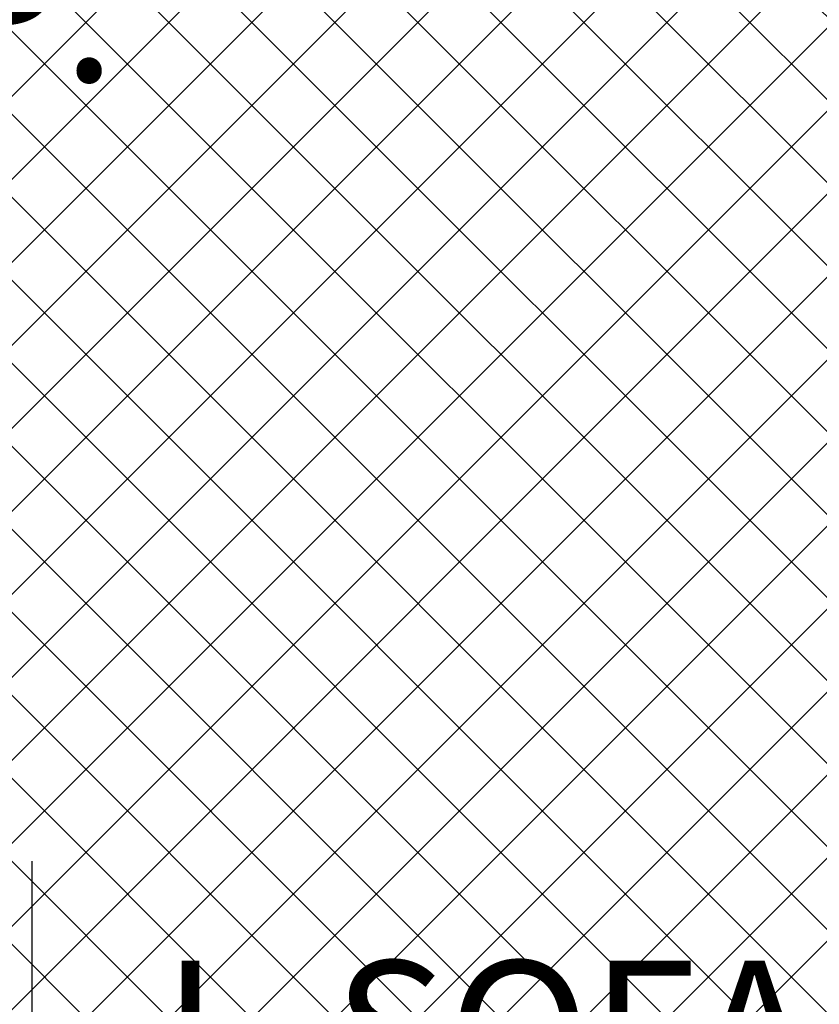
# Model space of a CAD drawing. Units: inches. Extents: x -466983 to 1020, y 324 to 318697.
# Tile 87 of 97: x 742 to 776, y 879 to 921. Entities that reach past the tile are written whole.
import ezdxf

# ---------------------------------------------------------------- set-up
doc = ezdxf.new("R2010")
doc.units = ezdxf.units.IN
doc.header["$MEASUREMENT"] = 0
doc.layers.add('A-ANNO-DIMS', color=2, linetype='Continuous', lineweight=18)
doc.layers.add('A-FLOR-PATT', color=252, linetype='Continuous', lineweight=13)
doc.styles.get("Standard").update_dxf_attribs({"font": 'arial.ttf'})
doc.dimstyles.get("Standard").update_dxf_attribs({"dimtxt": 6, "dimasz": 4, "dimexe": 3, "dimexo": 3, "dimgap": 0.09, "dimtad": 0, "dimtih": 1, "dimtoh": 1, "dimdec": 1, "dimzin": 0, "dimdsep": 46, "dimlunit": 3, "dimtxsty": 'Standard', "dimcen": 0.09, "dimadec": 0, "dimazin": 0, "dimtfac": 1, "dimtdec": 1, "dimtofl": 0, "dimtmove": 0, "dimatfit": 3, "dimfxl": 1, "dimtolj": 1, "dimtzin": 0, "dimarcsym": 0})

# ---------------------------------------------------------------- blocks, each defined once
blk = doc.blocks.new('*D71')
at = {"layer": 'A-ANNO-DIMS', "color": 0, "lineweight": -2, "transparency": 16777216}
for p, q in [((742.215, 885.152), (742.215, 874.91)), ((810.492, 885.152), (810.492, 874.91)), ((738.215, 877.91), (734.215, 877.91)), ((814.492, 877.91), (818.492, 877.91))]:
    blk.add_line(p, q, dxfattribs=at)
at = {"layer": 'A-ANNO-DIMS', "color": 0, "transparency": 16777216}
for points in [[(738.215, 878.577), (738.215, 877.244), (742.215, 877.91)], [(814.492, 878.577), (814.492, 877.244), (810.492, 877.91)]]:
    blk.add_solid(points, dxfattribs=at)
at = {"layer": 'Defpoints', "color": 0, "transparency": 16777216}
for p in [(742.215, 888.152), (810.492, 888.152), (742.215, 877.91)]:
    blk.add_point(p, dxfattribs=at)
at = {"layer": 'A-ANNO-DIMS', "color": 0, "transparency": 16777216, "insert": (776.354, 877.91), "char_height": 6, "attachment_point": 5}
blk.add_mtext('\\A1;L-SOFA 68 TYP.', dxfattribs=at)
blk = doc.blocks.new('*D72')
at = {"layer": 'A-ANNO-DIMS', "color": 0, "lineweight": -2, "transparency": 16777216}
for p, q in [((739.215, 954.575), (728.974, 954.575)), ((731.974, 950.575), (731.974, 924.517)), ((731.974, 892.152), (731.974, 918.21)), ((739.215, 888.152), (728.974, 888.152))]:
    blk.add_line(p, q, dxfattribs=at)
at = {"layer": 'A-ANNO-DIMS', "color": 0, "transparency": 16777216}
for points in [[(731.307, 950.575), (732.641, 950.575), (731.974, 954.575)], [(731.307, 892.152), (732.641, 892.152), (731.974, 888.152)]]:
    blk.add_solid(points, dxfattribs=at)
at = {"layer": 'Defpoints', "color": 0, "transparency": 16777216}
for p in [(731.974, 954.575), (742.215, 954.575), (742.215, 888.152)]:
    blk.add_point(p, dxfattribs=at)
at = {"layer": 'A-ANNO-DIMS', "color": 0, "transparency": 16777216, "insert": (731.974, 921.363), "char_height": 6, "attachment_point": 5}
blk.add_mtext('\\A1;66 TYP.', dxfattribs=at)

msp = doc.modelspace()

# ---------------------------------------------------------------- hatches: boundary and pattern name
at = {"layer": 'A-FLOR-PATT', "transparency": 33554572}
h = msp.add_hatch(dxfattribs=at)
h.set_pattern_fill('ANSI37', color=256, scale=30)
h.set_pattern_definition([(45, (-1212.4137, -290.035), (-2.6516504, 2.6516504), []), (135, (-1212.4137, -290.035), (-2.6516504, -2.6516504), [])])
h.paths.add_polyline_path([(901.806, 1075.938), (900.614, 1075.938), (900.614, 1065.386), (899.391, 1065.386), (898.091, 1065.386), (892.836, 1058.71, -0.258377), (892.188, 1058.351), (879.985, 1058.351, -0.20177), (879.438, 1058.581), (874.081, 1065.386), (872.781, 1065.386), (871.558, 1065.386), (871.558, 1075.938), (813.806, 1075.938), (813.806, 1044.792), (832.395, 1044.792, -0.394795), (848.66, 1028.536), (848.66, 1009.938), (901.806, 1009.938), (901.806, 1015.938), (901.306, 1015.938), (871.306, 1015.938), (871.306, 1017.25), (871.334, 1017.25, -0.401453), (901.306, 1045.938), (901.806, 1045.938)])
edge = h.paths.add_edge_path(flags=16)
edge.add_line((847.773, 1068.949), (847.773, 1073.709))
edge.add_arc((849.227, 1073.709), 1.454, 90, 180, ccw=False)
edge.add_line((849.227, 1075.163), (864.492, 1075.163))
edge.add_arc((864.492, 1073.709), 1.454, 0, 90, ccw=False)
edge.add_line((865.946, 1073.709), (865.946, 1069.004))
edge.add_arc((832.645, 1068.976), 33.301, -20.6123, 0.0472, ccw=False)
edge.add_ellipse((856.859, 1058.48), major_axis=(0, 10.213), ratio=0.685919, start_angle=100.0088, end_angle=259.9912, ccw=False)
edge.add_arc((881.074, 1068.976), 33.301, 180.0472, 200.6123, ccw=False)
h.paths.add_polyline_path([(853.146, 1066.482), (853.146, 1066.453), (853.146, 1066.453, 0.433107), (852.917, 1066.685), (852.917, 1066.453), (853.146, 1066.453), (853.146, 1066.482), (853.088, 1066.612, 0.697939), (852.7, 1066.453), (852.7, 1066.453), (852.7, 1066.482), (852.917, 1067.001), (852.917, 1066.685, -0.396254)], flags=0)
h.paths.add_polyline_path([(861.019, 1066.482), (861.019, 1066.453), (861.019, 1066.453, 0.416404), (860.802, 1066.685), (860.802, 1066.453), (861.019, 1066.453), (861.019, 1066.482), (860.967, 1066.605, 0.713344), (860.573, 1066.453), (860.573, 1066.453), (860.573, 1066.482), (860.802, 1067.001), (860.802, 1066.685, -0.379973)], flags=0)
edge = h.paths.add_edge_path(flags=0)
edge.add_spline(control_points=[(861.13, 1065.785), (861.466, 1065.248), (861.613, 1065.016), (861.983, 1064.374), (862.192, 1063.944), (862.561, 1063.039), (862.721, 1062.563), (862.987, 1061.578), (863.092, 1061.069), (863.245, 1060.031), (863.293, 1059.503), (863.329, 1058.441), (863.318, 1057.908), (863.237, 1056.852), (863.166, 1056.329), (862.97, 1055.308), (862.843, 1054.81), (862.537, 1053.852), (862.357, 1053.393), (861.951, 1052.525), (861.725, 1052.117), (861.233, 1051.362), (860.967, 1051.016), (860.405, 1050.395), (860.108, 1050.12), (859.494, 1049.646), (859.176, 1049.448), (858.528, 1049.13), (858.197, 1049.011), (857.531, 1048.852), (857.196, 1048.812), (856.525, 1048.812), (856.189, 1048.852), (855.524, 1049.01), (855.193, 1049.129), (854.545, 1049.447), (854.227, 1049.645), (853.612, 1050.118), (853.316, 1050.393), (852.753, 1051.014), (852.487, 1051.36), (851.995, 1052.114), (851.769, 1052.523), (851.363, 1053.39), (851.183, 1053.85), (850.877, 1054.807), (850.75, 1055.305), (850.553, 1056.326), (850.483, 1056.849), (850.401, 1057.905), (850.39, 1058.438), (850.426, 1059.5), (850.473, 1060.028), (850.626, 1061.066), (850.732, 1061.575), (850.997, 1062.561), (851.157, 1063.036), (851.525, 1063.942), (851.734, 1064.371), (852.106, 1065.016), (852.254, 1065.25), (852.608, 1065.733)], knot_values=[3.915332, 3.915332, 3.915332, 3.915332, 4.013468, 4.013468, 4.175532, 4.175532, 4.337596, 4.337596, 4.49966, 4.49966, 4.661724, 4.661724, 4.823788, 4.823788, 4.985852, 4.985852, 5.147916, 5.147916, 5.30998, 5.30998, 5.472044, 5.472044, 5.634109, 5.634109, 5.796173, 5.796173, 5.958237, 5.958237, 6.120301, 6.120301, 6.282365, 6.282365, 6.444429, 6.444429, 6.606493, 6.606493, 6.768557, 6.768557, 6.930621, 6.930621, 7.092685, 7.092685, 7.254749, 7.254749, 7.416813, 7.416813, 7.578878, 7.578878, 7.740942, 7.740942, 7.903006, 7.903006, 8.06507, 8.06507, 8.227134, 8.227134, 8.389198, 8.389198, 8.551262, 8.551262, 8.65037, 8.65037, 8.65037, 8.65037], degree=3, periodic=0)
edge.add_line((852.642, 1065.785), (861.13, 1065.785))
edge = h.paths.add_edge_path(flags=0)
edge.add_ellipse((856.85, 1057.743), major_axis=(0, 7.792), ratio=0.687861, start_angle=0, end_angle=360)
h.paths.add_polyline_path([(848.863, 1069.389), (848.863, 1073.96, -0.414214), (849.954, 1075.051), (863.765, 1075.051, -0.414214), (864.856, 1073.96), (864.856, 1069.389, -0.388936), (864.524, 1069.027, -0.043561), (849.195, 1069.027, -0.388936)], flags=0)
h.paths.add_polyline_path([(853.101, 1068.112, -1), (852.677, 1068.112, -1)], flags=0)
edge = h.paths.add_edge_path(flags=0)
edge.add_ellipse((856.859, 1057.338), major_axis=(0, 2.207), ratio=0.657164, start_angle=0, end_angle=360)
h.paths.add_polyline_path([(861.041, 1068.112, -1), (860.618, 1068.112, -1)], flags=0)
edge = h.paths.add_edge_path()
edge.add_line((573.954, 1057.341), (573.954, 1075.938))
edge.add_line((573.954, 1075.938), (558.731, 1075.938))
edge.add_line((558.731, 1075.938), (558.731, 1065.386))
edge.add_line((558.731, 1065.386), (557.507, 1065.386))
edge.add_line((557.507, 1065.386), (556.207, 1065.386))
edge.add_line((556.207, 1065.386), (550.952, 1058.71))
edge.add_arc((550.304, 1059.116), 0.765, 270, 327.9483, ccw=False)
edge.add_line((550.304, 1058.351), (538.101, 1058.351))
edge.add_arc((538.101, 1059.116), 0.765, 224.3704, 270, ccw=False)
edge.add_line((537.555, 1058.581), (532.198, 1065.386))
edge.add_line((532.198, 1065.386), (530.898, 1065.386))
edge.add_line((530.898, 1065.386), (529.674, 1065.386))
edge.add_line((529.674, 1065.386), (529.674, 1075.938))
edge.add_line((529.674, 1075.938), (520.806, 1075.938))
edge.add_line((520.806, 1075.938), (520.806, 1045.938))
edge.add_line((520.806, 1045.938), (521.306, 1045.938))
edge.add_arc((521.306, 1015.938), 30, 2.5075, 90, ccw=False)
edge.add_line((551.277, 1017.25), (551.306, 1017.25))
edge.add_line((551.306, 1017.25), (551.306, 1015.938))
edge.add_line((551.306, 1015.938), (520.806, 1015.938))
edge.add_line((520.806, 1015.938), (520.806, 1009.938))
edge.add_line((520.806, 1009.938), (559.191, 1010.402))
edge.add_arc((559.191, 1011.856), 1.454, 180, 270, ccw=False)
edge.add_line((557.737, 1011.856), (557.737, 1016.561))
edge.add_arc((591.039, 1016.589), 33.301, 159.3877, 180.0472, ccw=False)
edge.add_ellipse((566.824, 1027.085), major_axis=(0, 10.213), ratio=0.685919, start_angle=280.0088, end_angle=439.9912, ccw=False)
edge.add_arc((542.609, 1016.589), 33.301, 0.0472, 20.6123, ccw=False)
edge.add_line((575.91, 1016.616), (575.91, 1011.856))
edge.add_arc((574.456, 1011.856), 1.454, -90, 0, ccw=False)
edge.add_line((574.456, 1010.402), (608.806, 1009.938))
edge.add_line((608.806, 1009.938), (608.806, 1041.086))
edge.add_line((608.806, 1041.086), (590.218, 1041.086))
edge.add_arc((590.775, 1057.907), 16.831, 181.9277, 268.1032, ccw=False)
edge = h.paths.add_edge_path()
edge.add_ellipse((494.244, 583.62), major_axis=(0, 10.213), ratio=0.685919, start_angle=280.0088, end_angle=439.9912, ccw=False)
edge.add_arc((470.03, 573.124), 33.301, 0.0472, 20.6123, ccw=False)
edge.add_line((503.331, 573.152), (503.331, 568.392))
edge.add_arc((501.877, 568.392), 1.454, -90, 0, ccw=False)
edge.add_line((501.877, 566.938), (539.806, 566.938))
edge.add_line((539.806, 566.938), (539.806, 572.938))
edge.add_line((539.806, 572.938), (539.306, 572.938))
edge.add_line((539.306, 572.938), (509.306, 572.938))
edge.add_line((509.306, 572.938), (509.306, 574.25))
edge.add_line((509.306, 574.25), (509.334, 574.25))
edge.add_arc((539.306, 572.938), 30, 90, 177.4925, ccw=False)
edge.add_line((539.306, 602.938), (539.806, 602.938))
edge.add_line((539.806, 602.938), (539.806, 626.938))
edge.add_line((539.806, 626.938), (531.772, 626.938))
edge.add_line((531.772, 626.938), (531.772, 616.386))
edge.add_line((531.772, 616.386), (530.548, 616.386))
edge.add_line((530.548, 616.386), (529.249, 616.386))
edge.add_line((529.249, 616.386), (523.711, 609.351))
edge.add_line((523.711, 609.351), (510.777, 609.351))
edge.add_line((510.777, 609.351), (505.239, 616.386))
edge.add_line((505.239, 616.386), (503.939, 616.386))
edge.add_line((503.939, 616.386), (502.715, 616.386))
edge.add_line((502.715, 616.386), (502.715, 626.938))
edge.add_line((502.715, 626.938), (481.698, 626.938))
edge.add_line((481.698, 626.938), (481.698, 610.995))
edge.add_arc((467.27, 611.473), 14.436, 271.9277, 358.1032, ccw=False)
edge.add_line((467.756, 597.045), (451.806, 597.045))
edge.add_line((451.806, 597.045), (451.806, 584.404))
edge.add_line((451.806, 584.404), (451.806, 566.938))
edge.add_line((451.806, 566.938), (486.612, 566.938))
edge.add_arc((486.612, 568.392), 1.454, 180, 270, ccw=False)
edge.add_line((485.158, 568.392), (485.158, 573.097))
edge.add_arc((518.459, 573.124), 33.301, 159.3877, 180.0472, ccw=False)
h.paths.add_polyline_path([(836.261, 1020.733), (879.89, 1020.733), (879.89, 1039.39), (836.261, 1039.39)], flags=25)
h.paths.add_polyline_path([(549.985, 1036.749), (593.614, 1036.749), (593.614, 1055.407), (549.985, 1055.407)], flags=24)
h.paths.add_polyline_path([(475.123, 595.596), (518.752, 595.596), (518.752, 614.253), (475.123, 614.253)], flags=24)
h = msp.add_hatch(dxfattribs=at)
h.set_pattern_fill('ANSI37', color=256, scale=20)
h.set_pattern_definition([(45, (-1212.4137, -290.035), (-1.767767, 1.767767), []), (135, (-1212.4137, -290.035), (-1.767767, -1.767767), [])])
h.paths.add_polyline_path([(809.806, 870.938), (809.806, 888.152), (806.998, 888.152), (802.662, 888.152), (789.383, 888.152), (786.285, 888.152, -0.414214), (785.499, 888.937), (785.499, 900.196), (785.499, 908.47, -0.414214), (786.808, 909.779, -0.414214), (785.499, 911.088), (785.499, 929.101, -0.414214), (786.808, 930.411, -0.414214), (785.499, 931.72), (785.499, 931.904, -0.414214), (784.19, 930.595), (766.722, 930.595, -0.412359), (765.413, 931.896, -0.413741), (764.115, 930.578), (744.578, 930.422, -0.416556), (743.786, 931.207), (743.786, 933.515), (742.215, 933.515), (742.215, 952.024, -0.001344), (743.786, 952.2), (743.786, 953.938), (678.592, 953.938), (678.592, 951.131), (678.592, 946.794), (678.592, 933.515), (678.592, 930.417, -0.414214), (677.806, 929.631), (666.548, 929.631), (658.274, 929.631, -0.414214), (656.965, 930.94, -0.414214), (655.656, 929.631), (637.642, 929.631, -0.414214), (636.333, 930.94, -0.414214), (635.024, 929.631), (634.839, 929.631, -0.414214), (636.149, 928.322), (636.149, 910.854, -0.412359), (634.848, 909.545, -0.413741), (636.165, 908.247), (636.321, 888.71, -0.416556), (635.536, 887.918), (633.228, 887.918), (633.228, 886.347), (614.719, 886.347, -0.001344), (614.544, 887.918), (612.806, 887.918), (612.806, 834.938), (612.806, 752.938), (612.806, 748.938), (612.806, 697.938), (654.806, 697.938), (654.806, 701.938), (715.806, 701.938), (715.806, 737.435), (774.292, 737.435), (774.292, 795.938), (809.806, 795.938)])
h.paths.add_polyline_path([(679.276, 849.576, 0.102523), (682.148, 849.261, -0.080461), (694.543, 849.773, -0.283899), (694.482, 849.008, 0.136605), (694.407, 848.81, -0.030441), (694.543, 846.893), (694.543, 842.62), (694.543, 838.347, -0.028219), (694.425, 836.568), (694.425, 836.568, 0.196187), (694.446, 836.271, -0.302897), (694.543, 835.467, -0.080461), (682.148, 835.979, 0.102523), (679.276, 835.664, -0.58611), (678.646, 836.017), (678.646, 849.223, -0.58611)], flags=16)
h.paths.add_polyline_path([(679.517, 848.651, 0.699597), (679.476, 848.634, 1.20716), (679.194, 848.742, 0.010621)], flags=0)
h.paths.add_polyline_path([(679.492, 836.561, -0.013798), (679.918, 836.659, -0.071703), (682.853, 837.143, -0.165743), (682.166, 839.101), (682.166, 842.609), (682.166, 846.06, -0.240616), (683.473, 848.677, -0.068263), (693.929, 849.008), (693.788, 848.708), (693.788, 849.023, 0.067332), (683.473, 848.677, 0.240616), (682.166, 846.06), (682.166, 842.609), (682.166, 839.101, 0.23459), (683.461, 836.551, 0.068093), (693.788, 836.195), (693.788, 836.51), (693.93, 836.21, -0.077215), (682.242, 836.782, 0.086627), (679.528, 836.57, -0.628402), (679.503, 836.573), (679.503, 836.607, 0.910458)], flags=0)
h.paths.add_polyline_path([(679.476, 848.636), (679.207, 848.647), (679.207, 836.572, 0.913566), (679.365, 836.586), (679.476, 836.582)], flags=0)
h.paths.add_polyline_path([(679.276, 829.86, 0.102523), (682.148, 829.546, -0.080461), (694.543, 830.057, -0.283899), (694.482, 829.293, 0.136605), (694.407, 829.095, -0.030441), (694.543, 827.178), (694.543, 822.904), (694.543, 818.631, -0.028219), (694.425, 816.853), (694.425, 816.853, 0.196187), (694.446, 816.556, -0.302897), (694.543, 815.752, -0.080461), (682.148, 816.263, 0.102523), (679.276, 815.949, -0.58611), (678.646, 816.302), (678.646, 829.507, -0.58611)], flags=16)
h.paths.add_polyline_path([(679.517, 828.936, 0.699597), (679.476, 828.919, 1.20716), (679.194, 829.027, 0.010621)], flags=0)
h.paths.add_polyline_path([(679.492, 816.846, -0.013798), (679.918, 816.944, -0.071703), (682.853, 817.428, -0.165743), (682.166, 819.385), (682.166, 822.894), (682.166, 826.345, -0.240616), (683.473, 828.961, -0.068263), (693.929, 829.293), (693.788, 828.993), (693.788, 829.308, 0.067332), (683.473, 828.961, 0.240616), (682.166, 826.345), (682.166, 822.894), (682.166, 819.385, 0.23459), (683.461, 816.836, 0.068093), (693.788, 816.48), (693.788, 816.795), (693.93, 816.495, -0.077215), (682.242, 817.066, 0.086627), (679.528, 816.855, -0.628402), (679.503, 816.858), (679.503, 816.892, 0.910458)], flags=0)
h.paths.add_polyline_path([(679.476, 828.921), (679.207, 828.932), (679.207, 816.857, 0.913566), (679.365, 816.871), (679.476, 816.867)], flags=0)
h.paths.add_polyline_path([(679.276, 810.145, 0.102523), (682.148, 809.83, -0.080461), (694.543, 810.342, -0.3023), (694.447, 809.539, 0.10023), (694.406, 809.388, -0.03057), (694.543, 807.462), (694.543, 803.189), (694.543, 798.916, -0.03057), (694.406, 796.991, 0.10023), (694.447, 796.839, -0.3023), (694.543, 796.036, -0.080461), (682.148, 796.548, 0.102523), (679.276, 796.233, -0.58611), (678.646, 796.586), (678.646, 809.792, -0.58611)], flags=16)
h.paths.add_polyline_path([(679.517, 809.242, 0.699597), (679.476, 809.224, 1.20716), (679.194, 809.332, 0.010621)], flags=0)
h.paths.add_polyline_path([(679.492, 797.151, -0.013798), (679.918, 797.25, -0.071703), (682.853, 797.734, -0.165743), (682.166, 799.691), (682.166, 803.2), (682.166, 806.65, -0.239349), (683.461, 809.258, -0.072465), (694.447, 809.541, 0.197932), (694.425, 809.241), (693.788, 809.299), (693.788, 809.614, 0.068093), (683.461, 809.258, 0.239349), (682.166, 806.65), (682.166, 803.2), (682.166, 799.691, 0.235854), (683.473, 797.132, 0.067332), (693.788, 796.786), (693.788, 797.101), (694.425, 797.159, 0.197932), (694.447, 796.859, -0.080419), (682.156, 797.379, 0.083867), (679.528, 797.16, -0.628402), (679.503, 797.164), (679.503, 797.197, 0.910458)], flags=0)
h.paths.add_polyline_path([(679.207, 809.237), (679.207, 797.162, 0.913566), (679.365, 797.176), (679.476, 797.173), (679.476, 809.227)], flags=0)
h.paths.add_polyline_path([(695.364, 853.299), (728.223, 853.299), (728.223, 771.152), (695.364, 771.152)], flags=16)
h.paths.add_polyline_path([(696.021, 852.642), (727.566, 852.642), (727.566, 771.809), (696.021, 771.809)], flags=0)
h.paths.add_polyline_path([(679.276, 788.787, 0.102523), (682.148, 788.472, -0.080461), (694.543, 788.984, -0.3023), (694.447, 788.181, 0.10023), (694.406, 788.03, -0.03057), (694.543, 786.104), (694.543, 781.831), (694.543, 777.558, -0.03057), (694.406, 775.632, 0.10023), (694.447, 775.481, -0.3023), (694.543, 774.678, -0.080461), (682.148, 775.19, 0.102523), (679.276, 774.875, -0.58611), (678.646, 775.228), (678.646, 788.434, -0.58611)], flags=16)
h.paths.add_polyline_path([(679.517, 787.883, 0.699597), (679.476, 787.866, 1.20716), (679.194, 787.974, 0.010621)], flags=0)
h.paths.add_polyline_path([(679.492, 775.793, -0.013798), (679.918, 775.891, -0.071703), (682.853, 776.375, -0.165743), (682.166, 778.333), (682.166, 781.841), (682.166, 785.292, -0.239349), (683.461, 787.899, -0.072465), (694.447, 788.182, 0.197932), (694.425, 787.882), (693.788, 787.94), (693.788, 788.255, 0.068093), (683.461, 787.899, 0.239349), (682.166, 785.292), (682.166, 781.841), (682.166, 778.333, 0.235854), (683.473, 775.774, 0.067332), (693.788, 775.428), (693.788, 775.742), (694.425, 775.8, 0.197932), (694.447, 775.5, -0.080419), (682.156, 776.021, 0.083867), (679.528, 775.802, -0.628402), (679.503, 775.805), (679.503, 775.839, 0.910458)], flags=0)
h.paths.add_polyline_path([(679.207, 787.879), (679.207, 775.804, 0.913566), (679.365, 775.818), (679.476, 775.814), (679.476, 787.868)], flags=0)
h.paths.add_polyline_path([(704.641, 854.12, -0.080461), (705.153, 866.516, 0.102523), (704.838, 869.387, -0.58611), (705.191, 870.017), (718.397, 870.017, -0.58611), (718.75, 869.387, 0.102523), (718.435, 866.516, -0.080461), (718.946, 854.12, -0.3023), (718.144, 854.217, 0.10023), (717.992, 854.257, -0.03057), (716.067, 854.12), (711.794, 854.12), (707.521, 854.12, -0.03057), (705.595, 854.257, 0.10023), (705.444, 854.217, -0.3023)], flags=16)
h.paths.add_polyline_path([(717.846, 869.146, 0.699597), (717.829, 869.187, 1.20716), (717.937, 869.47, 0.010621)], flags=0)
h.paths.add_polyline_path([(705.463, 854.216, -0.080419), (705.984, 866.507, 0.083867), (705.765, 869.135, -0.628402), (705.768, 869.16), (705.802, 869.16, 0.910458), (705.756, 869.171, -0.013798), (705.854, 868.745, -0.071703), (706.338, 865.81, -0.165743), (708.295, 866.497), (711.804, 866.497), (715.255, 866.497, -0.239349), (717.862, 865.202, -0.072465), (718.145, 854.216, 0.197932), (717.845, 854.238), (717.903, 854.876), (718.218, 854.876, 0.068093), (717.862, 865.202, 0.239349), (715.255, 866.497), (711.804, 866.497), (708.295, 866.497, 0.235854), (705.737, 865.19, 0.067332), (705.391, 854.876), (705.705, 854.876), (705.763, 854.238, 0.197932)], flags=16)
h.paths.add_polyline_path([(705.766, 869.456, 0.913566), (705.781, 869.299), (705.777, 869.187), (717.831, 869.187), (717.842, 869.456)], flags=0)
h.paths.add_polyline_path([(729.045, 842.62), (729.045, 846.893, -0.03057), (729.182, 848.818, 0.10023), (729.141, 848.97, -0.3023), (729.045, 849.773, -0.080461), (741.44, 849.261, 0.102523), (744.311, 849.576, -0.58611), (744.942, 849.223), (744.942, 836.017, -0.58611), (744.311, 835.664, 0.102523), (741.44, 835.979, -0.080461), (729.045, 835.467, -0.3023), (729.141, 836.27, 0.10023), (729.182, 836.421, -0.03057), (729.045, 838.347)], flags=16)
h.paths.add_polyline_path([(744.111, 836.585, 1.20716), (744.394, 836.477, 0.010621), (744.07, 836.567, 0.699597)], flags=0)
h.paths.add_polyline_path([(729.141, 836.268, 0.197932), (729.162, 836.568), (729.8, 836.51), (729.8, 836.195, 0.068093), (740.126, 836.551, 0.239349), (741.421, 839.159), (741.421, 842.609), (741.421, 846.118, 0.235854), (740.114, 848.677, 0.067332), (729.8, 849.023), (729.8, 848.708), (729.162, 848.65, 0.197932), (729.141, 848.95, -0.080419), (741.432, 848.43, 0.083867), (744.059, 848.649, -0.628402), (744.085, 848.645), (744.085, 848.612, 0.910458), (744.095, 848.658, -0.013798), (743.67, 848.559, -0.071703), (740.734, 848.075, -0.165743), (741.421, 846.118), (741.421, 842.609), (741.421, 839.159, -0.239349), (740.126, 836.551, -0.072465)], flags=0)
h.paths.add_polyline_path([(729.045, 830.057, -0.080461), (741.44, 829.546, 0.102523), (744.311, 829.86, -0.58611), (744.942, 829.507), (744.942, 816.302, -0.58611), (744.311, 815.949, 0.102523), (741.44, 816.263, -0.080461), (729.045, 815.752, -0.3023), (729.141, 816.554, 0.10023), (729.182, 816.706, -0.03057), (729.045, 818.631), (729.045, 822.904), (729.045, 827.178, -0.03057), (729.182, 829.103, 0.10023), (729.141, 829.255, -0.3023)], flags=16)
h.paths.add_polyline_path([(744.111, 816.869, 1.20716), (744.394, 816.761, 0.010621), (744.07, 816.852, 0.699597)], flags=0)
h.paths.add_polyline_path([(729.141, 829.235, -0.080419), (741.432, 828.714, 0.083867), (744.059, 828.933, -0.628402), (744.085, 828.93), (744.085, 828.896, 0.910458), (744.095, 828.943, -0.013798), (743.67, 828.844, -0.071703), (740.734, 828.36, -0.165743), (741.421, 826.403), (741.421, 822.894), (741.421, 819.443, -0.239349), (740.126, 816.836, -0.072465), (729.141, 816.553, 0.197932), (729.162, 816.853), (729.8, 816.795), (729.8, 816.48, 0.068093), (740.126, 816.836, 0.239349), (741.421, 819.443), (741.421, 822.894), (741.421, 826.403, 0.235854), (740.114, 828.961, 0.067332), (729.8, 829.308), (729.8, 828.993), (729.162, 828.935, 0.197932)], flags=16)
h.paths.add_polyline_path([(729.045, 810.342, -0.080461), (741.44, 809.83, 0.102523), (744.311, 810.145, -0.58611), (744.942, 809.792), (744.942, 796.586, -0.58611), (744.311, 796.233, 0.102523), (741.44, 796.548, -0.080461), (729.045, 796.036, -0.283899), (729.105, 796.801, 0.136605), (729.181, 796.999, -0.030441), (729.045, 798.916), (729.045, 803.189), (729.045, 807.462, -0.028219), (729.163, 809.241), (729.162, 809.241, 0.196187), (729.142, 809.538, -0.302897)], flags=16)
h.paths.add_polyline_path([(744.111, 797.175, 1.20716), (744.394, 797.067, 0.010621), (744.07, 797.158, 0.699597)], flags=0)
h.paths.add_polyline_path([(741.345, 809.027, 0.086627), (744.059, 809.239, -0.628402), (744.085, 809.235), (744.085, 809.202, 0.910458), (744.095, 809.248, -0.013798), (743.67, 809.15, -0.071703), (740.734, 808.666, -0.165743), (741.421, 806.708), (741.421, 803.2), (741.421, 799.749, -0.240616), (740.114, 797.132, -0.068263), (729.658, 796.801), (729.8, 797.101), (729.8, 796.786, 0.067332), (740.114, 797.132, 0.240616), (741.421, 799.749), (741.421, 803.2), (741.421, 806.708, 0.23459), (740.126, 809.258, 0.068093), (729.8, 809.614), (729.8, 809.299), (729.658, 809.599, -0.077215)], flags=0)
h.paths.add_polyline_path([(704.641, 770.33, -0.283899), (705.405, 770.27, 0.136605), (705.603, 770.194, -0.030441), (707.521, 770.33), (711.794, 770.33), (716.067, 770.33, -0.028219), (717.845, 770.212), (717.845, 770.213, 0.196187), (718.143, 770.233, -0.302897), (718.946, 770.33, -0.080461), (718.435, 757.935, 0.102523), (718.75, 755.064, -0.58611), (718.397, 754.433), (705.191, 754.433, -0.58611), (704.838, 755.064, 0.102523), (705.153, 757.935, -0.080461)], flags=16)
h.paths.add_polyline_path([(705.762, 755.305, 0.699597), (705.779, 755.264, 1.20716), (705.671, 754.981, 0.010621)], flags=0)
h.paths.add_polyline_path([(705.405, 769.717), (705.705, 769.575), (705.391, 769.575, 0.067332), (705.737, 759.261, 0.240616), (708.353, 757.954), (711.804, 757.954), (715.313, 757.954, 0.23459), (717.862, 759.249, 0.068093), (718.218, 769.575), (717.903, 769.575), (718.203, 769.717, -0.077215), (717.632, 758.03, 0.086627), (717.843, 755.316, -0.628402), (717.84, 755.29), (717.806, 755.29, 0.910458), (717.853, 755.28, -0.013798), (717.754, 755.705, -0.071703), (717.27, 758.641, -0.165743), (715.313, 757.954), (711.804, 757.954), (708.353, 757.954, -0.240616), (705.737, 759.261, -0.068263)], flags=0)
h.paths.add_polyline_path([(729.045, 788.984, -0.080461), (741.44, 788.472, 0.102523), (744.311, 788.787, -0.58611), (744.942, 788.434), (744.942, 775.228, -0.58611), (744.311, 774.875, 0.102523), (741.44, 775.19, -0.080461), (729.045, 774.678, -0.283899), (729.105, 775.443, 0.136605), (729.181, 775.64, -0.030441), (729.045, 777.558), (729.045, 781.831), (729.045, 786.104, -0.028219), (729.163, 787.882), (729.162, 787.882, 0.196187), (729.142, 788.18, -0.302897)], flags=16)
h.paths.add_polyline_path([(744.111, 775.817, 1.20716), (744.394, 775.709, 0.010621), (744.07, 775.799, 0.699597)], flags=0)
h.paths.add_polyline_path([(741.345, 787.669, 0.086627), (744.059, 787.881, -0.628402), (744.085, 787.877), (744.085, 787.844, 0.910458), (744.095, 787.89, -0.013798), (743.67, 787.791, -0.071703), (740.734, 787.307, -0.165743), (741.421, 785.35), (741.421, 781.841), (741.421, 778.39, -0.240616), (740.114, 775.774, -0.068263), (729.658, 775.443), (729.8, 775.742), (729.8, 775.428, 0.067332), (740.114, 775.774, 0.240616), (741.421, 778.39), (741.421, 781.841), (741.421, 785.35, 0.23459), (740.126, 787.899, 0.068093), (729.8, 788.255), (729.8, 787.94), (729.658, 788.241, -0.077215)], flags=0)
h.paths.add_polyline_path([(744.111, 848.636), (744.111, 836.582), (744.381, 836.572), (744.381, 848.647, 0.913566), (744.223, 848.633)], flags=0)
h.paths.add_polyline_path([(744.223, 828.917), (744.111, 828.921), (744.111, 816.867), (744.381, 816.857), (744.381, 828.932, 0.913566)], flags=0)
h.paths.add_polyline_path([(717.831, 755.264), (705.777, 755.264), (705.766, 754.994), (717.842, 754.994, 0.913566), (717.827, 755.152)], flags=0)
h.paths.add_polyline_path([(744.223, 809.223), (744.111, 809.227), (744.111, 797.173), (744.381, 797.162), (744.381, 809.237, 0.913566)], flags=0)
h.paths.add_polyline_path([(744.111, 787.868), (744.111, 775.814), (744.381, 775.804), (744.381, 787.879, 0.913566), (744.223, 787.865)], flags=0)
h.paths.add_polyline_path([(678.877, 877.123), (737.613, 877.123), (737.613, 899.512), (678.877, 899.512)], flags=24)

# ---------------------------------------------------------------- dimensions: what is measured, and where the dimension line sits
at = {"layer": 'A-ANNO-DIMS'}
for base, p1, p2, angle, text, picture, middle in [((731.974, 954.575), (742.215, 888.152), (742.215, 954.575), 90, '<> TYP.', '*D72', (731.974, 921.363)), ((742.215, 877.91), (810.492, 888.152), (742.215, 888.152), 180, 'L-SOFA <> TYP.', '*D71', (776.354, 877.91))]:
    dim = msp.add_linear_dim(base=base, p1=p1, p2=p2, angle=angle, text=text, dimstyle='Standard', override={"dimdec": 0, "dimlfac": 1, "dimrnd": 0, "dimzin": 0, "dimdsep": 46, "dimlunit": 2}, dxfattribs=at)
    dim.commit()
    dim.dimension.update_dxf_attribs({"geometry": picture, "text_midpoint": middle})

doc.saveas('drawing.dxf')
